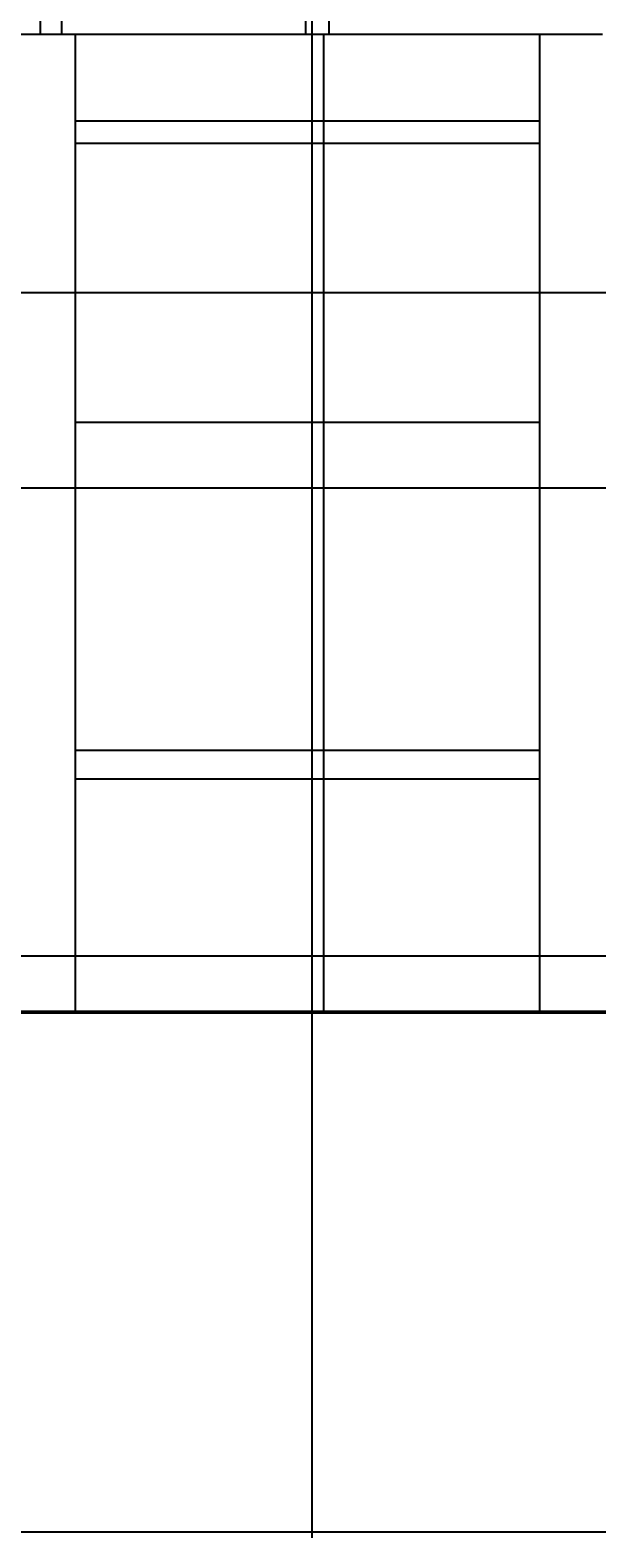
# Model space of a CAD drawing. Units: inches. Extents: x -117 to 121, y -77 to 40.
# Tile 18 of 45: x -23 to -6, y -77 to -32. Entities that reach past the tile are written whole.
import ezdxf

# ---------------------------------------------------------------- set-up
doc = ezdxf.new("R2010")
doc.units = ezdxf.units.IN
doc.header["$MEASUREMENT"] = 0
for name, color, linetype, lineweight in [('A-ANNO-DIMS', 2, 'Continuous', 18), ('A-ELEV', 7, 'Continuous', 25), ('A-ELEV-GRND', 7, 'Continuous', 50)]:
    doc.layers.add(name, color=color, linetype=linetype, lineweight=lineweight)
doc.styles.get("Standard").update_dxf_attribs({"font": 'arial.ttf'})
doc.dimstyles.get("Standard").update_dxf_attribs({"dimtxt": 0.18, "dimasz": 0.18, "dimexe": 0.18, "dimexo": 0.0625, "dimgap": 0.09, "dimtad": 0, "dimtih": 1, "dimtoh": 1, "dimdec": 4, "dimzin": 0, "dimdsep": 46, "dimtxsty": 'Standard', "dimcen": 0.09, "dimadec": 0, "dimazin": 0, "dimtfac": 1, "dimtdec": 4, "dimtofl": 0, "dimtmove": 0, "dimatfit": 3, "dimfxl": 1, "dimtolj": 1, "dimtzin": 0, "dimarcsym": 0})

# ---------------------------------------------------------------- blocks, each defined once
blk = doc.blocks.new('*D7')
at = {"layer": 'A-ANNO-DIMS', "color": 0, "lineweight": -2, "transparency": 16777216}
for p, q in [((-77.763, -61.431), (-77.763, -77.193)), ((90.549, -61.438), (90.549, -77.193)), ((-77.583, -77.013), (6.008, -77.013)), ((90.369, -77.013), (6.778, -77.013))]:
    blk.add_line(p, q, dxfattribs=at)
at = {"layer": 'A-ANNO-DIMS', "color": 0, "transparency": 16777216}
for points in [[(-77.583, -76.983), (-77.583, -77.043), (-77.763, -77.013)], [(90.369, -76.983), (90.369, -77.043), (90.549, -77.013)]]:
    blk.add_solid(points, dxfattribs=at)
at = {"layer": 'Defpoints', "color": 0, "transparency": 16777216}
for p in [(-77.763, -61.369), (90.549, -61.376), (90.549, -77.013)]:
    blk.add_point(p, dxfattribs=at)
at = {"layer": 'A-ANNO-DIMS', "color": 0, "transparency": 16777216, "insert": (6.393, -77.013), "char_height": 0.18, "attachment_point": 5}
blk.add_mtext('\\A1;168.3', dxfattribs=at)
blk = doc.blocks.new('*D13')
at = {"layer": 'A-ANNO-DIMS', "color": 0, "lineweight": -2, "transparency": 16777216}
for p, q in [((-2.663, 27.063), (-117.024, 27.063)), ((-116.844, 26.883), (-116.844, -16.974)), ((-116.844, -61.196), (-116.844, -17.338)), ((-106.096, -61.376), (-117.024, -61.376))]:
    blk.add_line(p, q, dxfattribs=at)
at = {"layer": 'A-ANNO-DIMS', "color": 0, "transparency": 16777216}
for points in [[(-116.874, 26.883), (-116.814, 26.883), (-116.844, 27.063)], [(-116.874, -61.196), (-116.814, -61.196), (-116.844, -61.376)]]:
    blk.add_solid(points, dxfattribs=at)
at = {"layer": 'Defpoints', "color": 0, "transparency": 16777216}
for p in [(-2.6, 27.063), (-116.844, -61.376), (-106.034, -61.376)]:
    blk.add_point(p, dxfattribs=at)
at = {"layer": 'A-ANNO-DIMS', "color": 0, "transparency": 16777216, "insert": (-116.844, -17.156), "char_height": 0.18, "attachment_point": 5}
blk.add_mtext('\\A1;88.44', dxfattribs=at)
blk = doc.blocks.new('*D37')
at = {"layer": 'A-ANNO-DIMS', "color": 0, "lineweight": -2, "transparency": 16777216}
for p, q in [((-3.912, -45.613), (-117.024, -45.613)), ((-116.844, -45.793), (-116.844, -52.47)), ((-116.844, -59.512), (-116.844, -52.834)), ((-3.912, -59.692), (-117.024, -59.692))]:
    blk.add_line(p, q, dxfattribs=at)
at = {"layer": 'A-ANNO-DIMS', "color": 0, "transparency": 16777216}
for points in [[(-116.874, -45.793), (-116.814, -45.793), (-116.844, -45.613)], [(-116.874, -59.512), (-116.814, -59.512), (-116.844, -59.692)]]:
    blk.add_solid(points, dxfattribs=at)
at = {"layer": 'Defpoints', "color": 0, "transparency": 16777216}
for p in [(-116.844, -45.613), (-3.85, -45.613), (-3.85, -59.692)]:
    blk.add_point(p, dxfattribs=at)
at = {"layer": 'A-ANNO-DIMS', "color": 0, "transparency": 16777216, "insert": (-116.844, -52.652), "char_height": 0.18, "attachment_point": 5}
blk.add_mtext('\\A1;14.079', dxfattribs=at)
blk = doc.blocks.new('*D49')
at = {"layer": 'A-ANNO-DIMS', "color": 0, "lineweight": -2, "transparency": 16777216}
for p, q in [((-45.422, -23.501), (120.84, -23.501)), ((120.66, -23.681), (120.66, -31.426)), ((120.66, -39.536), (120.66, -31.79)), ((-45.471, -39.716), (120.84, -39.716))]:
    blk.add_line(p, q, dxfattribs=at)
at = {"layer": 'A-ANNO-DIMS', "color": 0, "transparency": 16777216}
for points in [[(120.63, -23.681), (120.69, -23.681), (120.66, -23.501)], [(120.63, -39.536), (120.69, -39.536), (120.66, -39.716)]]:
    blk.add_solid(points, dxfattribs=at)
at = {"layer": 'Defpoints', "color": 0, "transparency": 16777216}
for p in [(-45.485, -23.501), (120.66, -23.501), (-45.533, -39.716)]:
    blk.add_point(p, dxfattribs=at)
at = {"layer": 'A-ANNO-DIMS', "color": 0, "transparency": 16777216, "insert": (120.66, -31.608), "char_height": 0.18, "attachment_point": 5}
blk.add_mtext('\\A1;16.215', dxfattribs=at)
blk = doc.blocks.new('*D56')
at = {"layer": 'A-ANNO-DIMS', "color": 0, "lineweight": -2, "transparency": 16777216}
for p, q in [((-14.23, -7.853), (-14.23, -77.193)), ((7.628, -8.105), (7.628, -77.193)), ((-14.05, -77.013), (-3.766, -77.013)), ((7.448, -77.013), (-2.835, -77.013))]:
    blk.add_line(p, q, dxfattribs=at)
at = {"layer": 'A-ANNO-DIMS', "color": 0, "transparency": 16777216}
for points in [[(-14.05, -76.983), (-14.05, -77.043), (-14.23, -77.013)], [(7.448, -76.983), (7.448, -77.043), (7.628, -77.013)]]:
    blk.add_solid(points, dxfattribs=at)
at = {"layer": 'Defpoints', "color": 0, "transparency": 16777216}
for p in [(-14.23, -7.791), (7.628, -8.042), (7.628, -77.013)]:
    blk.add_point(p, dxfattribs=at)
at = {"layer": 'A-ANNO-DIMS', "color": 0, "transparency": 16777216, "insert": (-3.301, -77.013), "char_height": 0.18, "attachment_point": 5}
blk.add_mtext('\\A1;21.858', dxfattribs=at)

msp = doc.modelspace()

# ---------------------------------------------------------------- linework, layer by layer
at = {"layer": 'A-ELEV'}
for p, q in [((-21.7693, -15.0526), (-21.7693, -31.9617)), ((-14.4219, -15.0526), (-14.4219, -31.9617)), ((-22.4056, -24.6358), (-22.4056, -31.9617)), ((-13.7272, -29.1126), (-13.7272, -31.9617)), ((-5.4823, -31.9617), (-35.7647, -31.9617)), ((-21.3417, -45.6125), (-21.3417, -31.9617)), ((-13.886, -31.9617), (-13.886, -61.3756)), ((-7.3727, -45.6125), (-7.3727, -31.9617)), ((-7.3727, -34.5666), (-21.3417, -34.5666)), ((-7.3727, -35.2347), (-21.3417, -35.2347)), ((-7.3727, -43.6334), (-21.3417, -43.6334)), ((-7.3727, -45.6125), (-21.3417, -45.6125)), ((-21.3417, -61.3756), (-21.3417, -45.6125)), ((-7.3727, -61.3756), (-7.3727, -45.6125)), ((-7.3727, -53.5071), (-21.3417, -53.5071)), ((-7.3727, -54.3632), (-21.3417, -54.3632))]:
    msp.add_line(p, q, dxfattribs=at)
at = {"layer": 'A-ELEV-GRND'}
msp.add_line((90.5486, -61.3756), (-87.9273, -61.3756), dxfattribs=at)

# ---------------------------------------------------------------- dimensions: what is measured, and where the dimension line sits
at = {"layer": 'A-ANNO-DIMS'}
for base, p1, p2, override, picture, middle in [((-116.8438, -61.3756), (-2.6001, 27.0634), (-106.0338, -61.3756), {"dimdec": 2, "dimlfac": 1, "dimrnd": 0, "dimzin": 0, "dimdsep": 46, "dimlunit": 2}, '*D13', (-116.8438, -17.1561)), ((120.6602, -23.5007), (-45.5331, -39.716), (-45.4848, -23.5007), {"dimdec": 3, "dimlfac": 1, "dimrnd": 0, "dimzin": 0, "dimdsep": 46, "dimlunit": 2}, '*D49', (120.6602, -31.6083)), ((-116.843772, -45.612514), (-3.849514, -59.692012), (-3.849514, -45.612514), {"dimdec": 3, "dimlfac": 1, "dimrnd": 0, "dimzin": 0, "dimdsep": 46, "dimlunit": 2}, '*D37', (-116.843772, -52.652263))]:
    dim = msp.add_linear_dim(base=base, p1=p1, p2=p2, angle=90, dimstyle='Standard', override=override, dxfattribs=at)
    dim.commit()
    dim.dimension.update_dxf_attribs({"geometry": picture, "text_midpoint": middle})
for base, p1, p2, override, picture, middle in [((7.6284, -77.0135), (-14.2298, -7.7907), (7.6284, -8.0421), {"dimdec": 3, "dimlfac": 1, "dimrnd": 0, "dimzin": 0, "dimdsep": 46, "dimlunit": 2}, '*D56', (-3.3007, -77.0135)), ((90.5486, -77.0135), (-77.7631, -61.3689), (90.5486, -61.3756), {"dimdec": 1, "dimlfac": 1, "dimrnd": 0, "dimzin": 0, "dimdsep": 46, "dimlunit": 2}, '*D7', (6.3928, -77.0135))]:
    dim = msp.add_linear_dim(base=base, p1=p1, p2=p2, dimstyle='Standard', override=override, dxfattribs=at)
    dim.commit()
    dim.dimension.update_dxf_attribs({"geometry": picture, "text_midpoint": middle})

doc.saveas('drawing.dxf')
